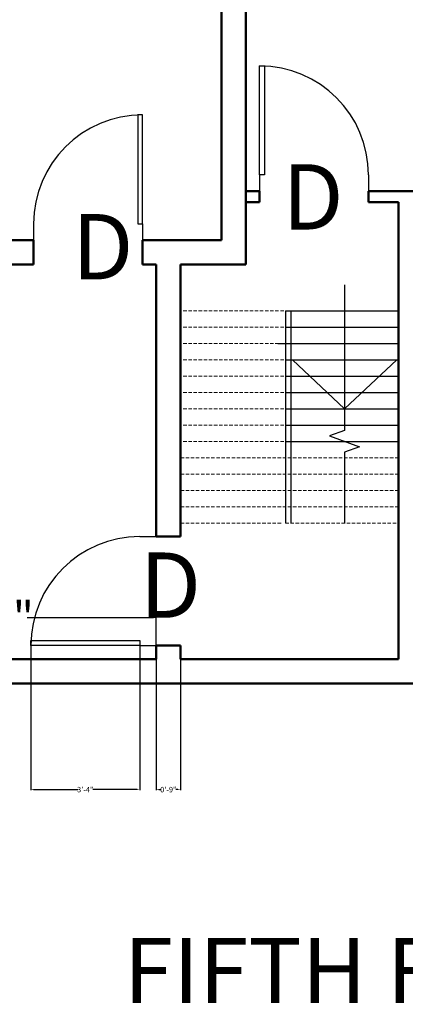
# Model space of a CAD drawing. Units: inches. Extents: x 409 to 7572, y 7 to 725.
# Tile 35 of 38: x 7079 to 7221, y 39 to 401. Entities that reach past the tile are written whole.
import ezdxf

# ---------------------------------------------------------------- set-up
doc = ezdxf.new("R2010")
doc.units = ezdxf.units.IN
doc.header["$MEASUREMENT"] = 0
doc.linetypes.add('HIDDEN', pattern=[0.375, 0.25, -0.125])
for name, color, linetype, lineweight in [('A-ANNO-DIMS', 2, 'Continuous', 18), ('A-ANNO-SYMB', 3, 'Continuous', 25), ('A-ANNO-TEXT', 7, 'Continuous', 35), ('A-DOOR', 3, 'Continuous', 25), ('A-FLOR-STRS', 6, 'Continuous', 25), ('A-FLOR-STRS-OVHD', 6, 'HIDDEN', 18), ('A-WALL', 7, 'Continuous', 50)]:
    doc.layers.add(name, color=color, linetype=linetype, lineweight=lineweight)
doc.styles.get("Standard").update_dxf_attribs({"font": 'arial.ttf'})
doc.dimstyles.get("Standard").update_dxf_attribs({"dimtxt": 2, "dimasz": 1, "dimexe": 0.18, "dimexo": 0.0625, "dimgap": 0.09, "dimtad": 0, "dimtih": 1, "dimtoh": 1, "dimdec": 0, "dimzin": 0, "dimdsep": 46, "dimlunit": 3, "dimtxsty": 'Standard', "dimcen": 0.09, "dimadec": 0, "dimazin": 0, "dimtfac": 1, "dimtdec": 0, "dimtofl": 0, "dimtmove": 0, "dimatfit": 3, "dimfxl": 1, "dimtolj": 1, "dimtzin": 0, "dimarcsym": 0})

# ---------------------------------------------------------------- blocks, each defined once
blk = doc.blocks.new('*U2')
for p, q in [((0, 0), (0, -6)), ((-40, 0), (-40, -6))]:
    blk.add_line(p, q)
blk.add_lwpolyline([(0, 0), (0, 40), (-1.75, 40), (-1.75, 0)], close=True)
blk.add_arc((0, 0), 40, 90, 180)
blk = doc.blocks.new('*U3')
for p, q in [((0, 0), (0, -6)), ((40, 0), (40, -6))]:
    blk.add_line(p, q)
blk.add_lwpolyline([(0, 0), (0, 40), (1.75, 40), (1.75, 0)], close=True)
blk.add_arc((0, 0), 40, 0, 90)
blk = doc.blocks.new('*U4')
for p, q in [((0, 0), (0, -6)), ((40, 0), (40, -6))]:
    blk.add_line(p, q)
blk.add_lwpolyline([(0, 0), (0, 40), (1.75, 40), (1.75, 0)], close=True)
blk.add_arc((0, 0), 40, 0, 90)
blk = doc.blocks.new('*D150')
at = {"layer": 'A-ANNO-DIMS', "color": 0, "lineweight": -2, "transparency": 16777216}
for p, q in [((6994.41, 165.59), (6994.41, 180.91)), ((6995.41, 180.73), (7041.78, 180.73)), ((7128.41, 180.73), (7082.05, 180.73)), ((7129.41, 165.59), (7129.41, 180.91))]:
    blk.add_line(p, q, dxfattribs=at)
at = {"layer": 'A-ANNO-DIMS', "color": 0, "transparency": 16777216}
for points in [[(6995.41, 180.9), (6995.41, 180.56), (6994.41, 180.73)], [(7128.41, 180.9), (7128.41, 180.56), (7129.41, 180.73)]]:
    blk.add_solid(points, dxfattribs=at)
at = {"layer": 'DEFPOINTS', "color": 0, "transparency": 16777216}
for p in [(7129.41, 180.73), (6994.41, 165.53), (7129.41, 165.53)]:
    blk.add_point(p, dxfattribs=at)
at = {"layer": 'A-ANNO-DIMS', "color": 0, "transparency": 16777216, "insert": (7061.91, 180.73), "char_height": 2, "attachment_point": 5}
blk.add_mtext('\\A1;{\\H6x;11\'-3"}', dxfattribs=at)
blk = doc.blocks.new('*D198')
at = {"layer": 'A-ANNO-DIMS', "color": 0, "lineweight": -2, "transparency": 16777216}
for p, q in [((7129.41, 165.47), (7129.41, 117.35)), ((7138.41, 165.47), (7138.41, 117.35)), ((7130.41, 117.53), (7131.16, 117.53)), ((7137.41, 117.53), (7136.66, 117.53))]:
    blk.add_line(p, q, dxfattribs=at)
at = {"layer": 'A-ANNO-DIMS', "color": 0, "transparency": 16777216}
for points in [[(7130.41, 117.7), (7130.41, 117.36), (7129.41, 117.53)], [(7137.41, 117.7), (7137.41, 117.36), (7138.41, 117.53)]]:
    blk.add_solid(points, dxfattribs=at)
at = {"layer": 'DEFPOINTS', "color": 0, "transparency": 16777216}
for p in [(7129.41, 165.53), (7138.41, 165.53), (7138.41, 117.53)]:
    blk.add_point(p, dxfattribs=at)
at = {"layer": 'A-ANNO-DIMS', "color": 0, "transparency": 16777216, "insert": (7133.91, 117.53), "char_height": 2, "attachment_point": 5}
blk.add_mtext('\\A1;0\'-9"', dxfattribs=at)
blk = doc.blocks.new('*D199')
at = {"layer": 'A-ANNO-DIMS', "color": 0, "lineweight": -2, "transparency": 16777216}
for p, q in [((7083.41, 170.47), (7083.41, 117.35)), ((7123.41, 170.47), (7123.41, 117.35)), ((7084.41, 117.53), (7100.66, 117.53)), ((7122.41, 117.53), (7106.16, 117.53))]:
    blk.add_line(p, q, dxfattribs=at)
at = {"layer": 'A-ANNO-DIMS', "color": 0, "transparency": 16777216}
for points in [[(7084.41, 117.7), (7084.41, 117.36), (7083.41, 117.53)], [(7122.41, 117.7), (7122.41, 117.36), (7123.41, 117.53)]]:
    blk.add_solid(points, dxfattribs=at)
at = {"layer": 'DEFPOINTS', "color": 0, "transparency": 16777216}
for p in [(7083.41, 170.53), (7123.41, 170.53), (7123.41, 117.53)]:
    blk.add_point(p, dxfattribs=at)
at = {"layer": 'A-ANNO-DIMS', "color": 0, "transparency": 16777216, "insert": (7103.41, 117.53), "char_height": 2, "attachment_point": 5}
blk.add_mtext('\\A1;3\'-4"', dxfattribs=at)

msp = doc.modelspace()

# ---------------------------------------------------------------- linework, layer by layer
at = {"layer": 'A-FLOR-STRS'}
for p, q in [((7198.62, 303.06), (7198.62, 257.53)), ((7176.91, 293.53), (7218.41, 293.53)), ((7176.91, 293.53), (7176.91, 215.53)), ((7178.91, 293.53), (7178.91, 215.53)), ((7176.91, 287.53), (7218.41, 287.53)), ((7174.07, 281.53), (7218.41, 281.53)), ((7176.91, 275.53), (7218.41, 275.53)), ((7198.62, 257.53), (7179.49, 275.53)), ((7198.62, 257.53), (7217.75, 275.53)), ((7176.91, 269.53), (7218.41, 269.53)), ((7176.91, 263.53), (7218.41, 263.53)), ((7176.91, 257.53), (7218.41, 257.53)), ((7176.91, 251.53), (7218.41, 251.53)), ((7176.91, 245.53), (7218.41, 245.53))]:
    msp.add_line(p, q, dxfattribs=at)
msp.add_lwpolyline([(7198.62, 257.71), (7198.62, 249.53), (7193.12, 247.53), (7204.11, 243.53), (7198.62, 241.53), (7198.62, 215.35)], dxfattribs=at)
at = {"layer": 'A-FLOR-STRS-OVHD', "ltscale": 5}
for p, q in [((7139.41, 293.53), (7176.91, 293.53)), ((7139.41, 287.53), (7176.91, 287.53)), ((7139.41, 281.53), (7174.07, 281.53)), ((7139.41, 275.53), (7176.91, 275.53)), ((7139.41, 269.53), (7176.91, 269.53)), ((7139.41, 263.53), (7176.91, 263.53)), ((7139.41, 257.53), (7176.91, 257.53)), ((7139.41, 251.53), (7176.91, 251.53)), ((7139.41, 245.53), (7176.91, 245.53)), ((7138.41, 239.53), (7218.41, 239.53)), ((7138.41, 233.53), (7218.41, 233.53)), ((7138.41, 227.53), (7218.41, 227.53)), ((7138.41, 221.53), (7218.41, 221.53)), ((7138.41, 215.53), (7175.91, 215.53)), ((7176.91, 215.53), (7218.41, 215.53))]:
    msp.add_line(p, q, dxfattribs=at)
at = {"layer": 'A-WALL'}
for p, q in [((7162.41, 663.53), (7162.41, 337.53)), ((7153.41, 525.53), (7153.41, 319.53)), ((7162.41, 337.53), (7167.41, 337.53)), ((7162.41, 337.53), (7162.41, 333.53)), ((7167.41, 337.53), (7167.41, 333.53)), ((7207.41, 337.53), (7228.41, 337.53)), ((7207.41, 337.53), (7207.41, 333.53)), ((7162.41, 333.53), (7167.41, 333.53)), ((7162.41, 333.53), (7162.41, 310.53)), ((7207.41, 333.53), (7218.41, 333.53)), ((7218.41, 333.53), (7218.41, 165.53)), ((7084.41, 319.53), (7034.41, 319.53)), ((7084.41, 319.53), (7084.41, 310.53)), ((7153.41, 319.53), (7124.41, 319.53)), ((7124.41, 310.53), (7124.41, 319.53)), ((7084.41, 310.53), (6994.41, 310.53)), ((7129.41, 310.53), (7124.41, 310.53)), ((7129.41, 310.53), (7129.41, 210.53)), ((7162.41, 310.53), (7138.41, 310.53)), ((7138.41, 310.53), (7138.41, 210.53)), ((7129.41, 210.53), (7138.41, 210.53)), ((7129.41, 170.53), (7129.41, 165.53)), ((7138.41, 170.53), (7129.41, 170.53)), ((7138.41, 170.53), (7138.41, 165.53)), ((6994.41, 165.53), (7129.41, 165.53)), ((7138.41, 165.53), (7218.41, 165.53)), ((6985.41, 156.53), (7359.41, 156.53))]:
    msp.add_line(p, q, dxfattribs=at)

# ---------------------------------------------------------------- block references
at = {"layer": 'A-DOOR'}
for name, p in [('*U4', (7167.41, 343.53)), ('*U2', (7124.41, 325.53))]:
    msp.add_blockref(name, p, dxfattribs=at)
at = {"layer": 'A-DOOR', "rotation": 90}
msp.add_blockref('*U3', (7123.41, 170.53), dxfattribs=at)

# ---------------------------------------------------------------- texts
at = {"layer": 'A-ANNO-SYMB', "char_height": 24, "attachment_point": 1}
for insert in [(7175.71, 347.4), (7098.55, 329.09), (7123.41, 204.69)]:
    msp.add_mtext_dynamic_manual_height_columns('D', width=19.1972, gutter_width=1, heights=[0], dxfattribs=dict(at, insert=insert))
at = {"layer": 'A-ANNO-TEXT', "insert": (7117.54, 63.03), "char_height": 24, "attachment_point": 1}
msp.add_mtext_dynamic_manual_height_columns('FIFTH FLOOR', width=577.2242, gutter_width=1, heights=[0], dxfattribs=at)

# ---------------------------------------------------------------- dimensions: what is measured, and where the dimension line sits
at = {"layer": 'A-ANNO-DIMS'}
dim = msp.add_linear_dim(base=(7129.41, 180.73), p1=(6994.41, 165.53), p2=(7129.41, 165.53), text='{\\H6x;<>}', dimstyle='Standard', override={"dimclrd": 0, "dimclre": 0, "dimclrt": 0}, dxfattribs=at)
dim.commit()
dim.dimension.update_dxf_attribs({"geometry": '*D150', "text_midpoint": (7061.91, 180.73)})
for base, p1, p2, picture, middle in [((7123.41, 117.53), (7083.41, 170.53), (7123.41, 170.53), '*D199', (7103.41, 117.53)), ((7138.41, 117.53), (7129.41, 165.53), (7138.41, 165.53), '*D198', (7133.91, 117.53))]:
    dim = msp.add_linear_dim(base=base, p1=p1, p2=p2, dimstyle='Standard', override={"dimdec": 1, "dimlfac": 1, "dimrnd": 0, "dimzin": 1, "dimdsep": 46, "dimlunit": 4, "dimfrac": 2}, dxfattribs=at)
    dim.commit()
    dim.dimension.update_dxf_attribs({"geometry": picture, "text_midpoint": middle})

doc.saveas('drawing.dxf')
